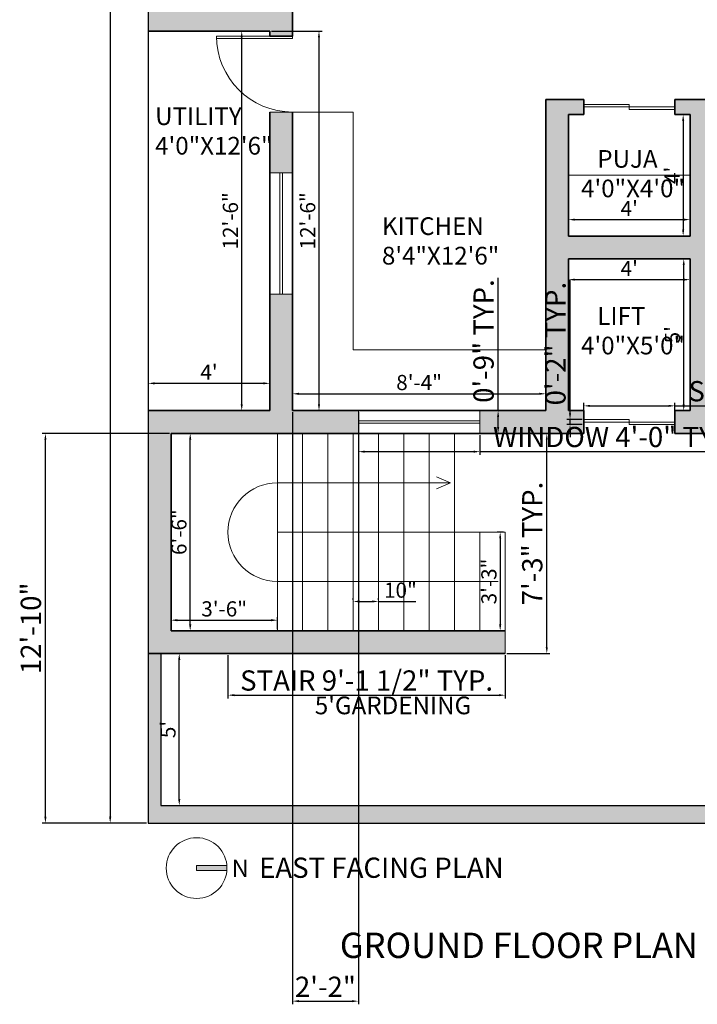
# Model space of a CAD drawing. Units: inches. Extents: x 2700 to 4052, y 1030 to 1872.
# Tile 5 of 8: x 3518 to 3786, y 1030 to 1419. Entities that reach past the tile are written whole.
import ezdxf

# ---------------------------------------------------------------- set-up
doc = ezdxf.new("R2010")
doc.units = ezdxf.units.IN
for name, color, linetype, lineweight in [('A-ANNO-DIMS', 2, 'Continuous', 13), ('A-ANNO-SYMB', 7, 'Continuous', 18), ('A-ANNO-TITL', 7, 'Continuous', 25), ('A-AREA-IDEN', 7, 'Continuous', 18), ('A-DOOR', 4, 'Continuous', 18), ('A-FLOR-CASE', 8, 'Continuous', 18), ('A-FLOR-STRS', 7, 'Continuous', 18), ('A-GLAZ', 4, 'Continuous', 18), ('A-WALL', 7, 'Continuous', 35), ('A-WALL-PATT', 7, 'Continuous', 13), ('C-PROP', 7, 'Continuous', 25)]:
    doc.layers.add(name, color=color, linetype=linetype, lineweight=lineweight)
doc.layers.add('C-SITE-PATT', color=252, linetype='Continuous', lineweight=13, true_color=0x939598)
doc.styles.get("Standard").update_dxf_attribs({"font": 'arial.ttf'})
doc.dimstyles.new('ISO-25', dxfattribs={"dimtxt": 8, "dimasz": 2.5, "dimexe": 1.25, "dimexo": 0.625, "dimtad": 1, "dimdec": 1, "dimlunit": 3, "dimtxsty": 'Standard', "dimcen": 2.5, "dimclrt": 1, "dimadec": 0, "dimazin": 0, "dimtfac": 1, "dimtdec": 1, "dimtmove": 0, "dimatfit": 3, "dimfxl": 1, "dimarcsym": 0})

# ---------------------------------------------------------------- blocks, each defined once
blk = doc.blocks.new('*D22')
at = {"layer": 'A-ANNO-DIMS', "color": 0, "lineweight": -2, "transparency": 16777216}
for p, q in [((3568.26, 1821.52), (3552.61, 1821.52)), ((3553.86, 1819.02), (3553.86, 1104.02)), ((3568.26, 1101.52), (3552.61, 1101.52))]:
    blk.add_line(p, q, dxfattribs=at)
at = {"layer": 'A-ANNO-DIMS', "color": 0, "transparency": 16777216}
for points in [[(3553.44, 1819.02), (3554.28, 1819.02), (3553.86, 1821.52)], [(3553.44, 1104.02), (3554.28, 1104.02), (3553.86, 1101.52)]]:
    blk.add_solid(points, dxfattribs=at)
at = {"layer": 'Defpoints', "color": 0, "transparency": 16777216}
for p in [(3568.88, 1821.52), (3553.86, 1101.52), (3568.88, 1101.52)]:
    blk.add_point(p, dxfattribs=at)
at = {"layer": 'A-ANNO-DIMS', "color": 0, "transparency": 16777216, "insert": (3549.15, 1461.52), "char_height": 8, "attachment_point": 5, "rotation": 90}
blk.add_mtext("60'", dxfattribs=at)
blk = doc.blocks.new('*D23')
at = {"layer": 'A-ANNO-DIMS', "color": 0, "lineweight": -2, "transparency": 16777216}
for p, q in [((3578.51, 1255.52), (3586.72, 1255.52)), ((3585.47, 1180.02), (3585.47, 1253.02)), ((3578.51, 1177.52), (3586.72, 1177.52))]:
    blk.add_line(p, q, dxfattribs=at)
at = {"layer": 'A-ANNO-DIMS', "color": 0, "transparency": 16777216}
for points in [[(3585.05, 1253.02), (3585.89, 1253.02), (3585.47, 1255.52)], [(3585.05, 1180.02), (3585.89, 1180.02), (3585.47, 1177.52)]]:
    blk.add_solid(points, dxfattribs=at)
at = {"layer": 'Defpoints', "color": 0, "transparency": 16777216}
for p in [(3577.88, 1255.52), (3585.47, 1255.52), (3577.88, 1177.52)]:
    blk.add_point(p, dxfattribs=at)
at = {"layer": 'A-ANNO-DIMS', "color": 0, "transparency": 16777216, "insert": (3581.78, 1216.52), "char_height": 6, "attachment_point": 5, "rotation": 90}
blk.add_mtext('6\'-6"', dxfattribs=at)
blk = doc.blocks.new('*D24')
at = {"layer": 'A-ANNO-DIMS', "color": 0, "lineweight": -2, "transparency": 16777216}
for p, q in [((3577.88, 1178.14), (3577.88, 1182.97)), ((3619.88, 1178.14), (3619.88, 1182.97)), ((3580.38, 1181.72), (3617.38, 1181.72))]:
    blk.add_line(p, q, dxfattribs=at)
at = {"layer": 'A-ANNO-DIMS', "color": 0, "transparency": 16777216}
for points in [[(3580.38, 1182.14), (3580.38, 1181.3), (3577.88, 1181.72)], [(3617.38, 1182.14), (3617.38, 1181.3), (3619.88, 1181.72)]]:
    blk.add_solid(points, dxfattribs=at)
at = {"layer": 'Defpoints', "color": 0, "transparency": 16777216}
for p in [(3619.88, 1181.72), (3577.88, 1177.52), (3619.88, 1177.52)]:
    blk.add_point(p, dxfattribs=at)
at = {"layer": 'A-ANNO-DIMS', "color": 0, "transparency": 16777216, "insert": (3598.88, 1185.41), "char_height": 6, "attachment_point": 5}
blk.add_mtext('3\'-6"', dxfattribs=at)
blk = doc.blocks.new('*D25')
at = {"layer": 'A-ANNO-DIMS', "color": 0, "lineweight": -2, "transparency": 16777216}
for p, q in [((3649.88, 1189.74), (3649.88, 1190.37)), ((3652.38, 1189.12), (3657.38, 1189.12)), ((3659.88, 1189.74), (3659.88, 1190.37)), ((3659.88, 1189.12), (3674.63, 1189.12))]:
    blk.add_line(p, q, dxfattribs=at)
at = {"layer": 'A-ANNO-DIMS', "color": 0, "transparency": 16777216}
for points in [[(3652.38, 1189.54), (3652.38, 1188.7), (3649.88, 1189.12)], [(3657.38, 1189.54), (3657.38, 1188.7), (3659.88, 1189.12)]]:
    blk.add_solid(points, dxfattribs=at)
at = {"layer": 'Defpoints', "color": 0, "transparency": 16777216}
for p in [(3649.88, 1189.12), (3659.88, 1189.12), (3659.88, 1189.12)]:
    blk.add_point(p, dxfattribs=at)
at = {"layer": 'A-ANNO-DIMS', "color": 0, "transparency": 16777216, "insert": (3668.5, 1192.81), "char_height": 6, "attachment_point": 5}
blk.add_mtext('10"', dxfattribs=at)
blk = doc.blocks.new('*D26')
at = {"layer": 'A-ANNO-DIMS', "color": 0, "lineweight": -2, "transparency": 16777216}
for p, q in [((3709.26, 1216.52), (3706.66, 1216.52)), ((3707.91, 1214.02), (3707.91, 1180.02)), ((3709.26, 1177.52), (3706.66, 1177.52))]:
    blk.add_line(p, q, dxfattribs=at)
at = {"layer": 'A-ANNO-DIMS', "color": 0, "transparency": 16777216}
for points in [[(3707.49, 1214.02), (3708.32, 1214.02), (3707.91, 1216.52)], [(3707.49, 1180.02), (3708.32, 1180.02), (3707.91, 1177.52)]]:
    blk.add_solid(points, dxfattribs=at)
at = {"layer": 'Defpoints', "color": 0, "transparency": 16777216}
for p in [(3709.88, 1216.52), (3707.91, 1177.52), (3709.88, 1177.52)]:
    blk.add_point(p, dxfattribs=at)
at = {"layer": 'A-ANNO-DIMS', "color": 0, "transparency": 16777216, "insert": (3704.22, 1197.02), "char_height": 6, "attachment_point": 5, "rotation": 90}
blk.add_mtext('3\'-3"', dxfattribs=at)
blk = doc.blocks.new('*D27')
at = {"layer": 'A-ANNO-DIMS', "color": 0, "lineweight": -2, "transparency": 16777216}
for p, q in [((3574.51, 1168.52), (3582.39, 1168.52)), ((3581.14, 1111.02), (3581.14, 1166.02)), ((3574.51, 1108.52), (3582.39, 1108.52))]:
    blk.add_line(p, q, dxfattribs=at)
at = {"layer": 'A-ANNO-DIMS', "color": 0, "transparency": 16777216}
for points in [[(3580.72, 1166.02), (3581.56, 1166.02), (3581.14, 1168.52)], [(3580.72, 1111.02), (3581.56, 1111.02), (3581.14, 1108.52)]]:
    blk.add_solid(points, dxfattribs=at)
at = {"layer": 'Defpoints', "color": 0, "transparency": 16777216}
for p in [(3573.88, 1168.52), (3581.14, 1168.52), (3573.88, 1108.52)]:
    blk.add_point(p, dxfattribs=at)
at = {"layer": 'A-ANNO-DIMS', "color": 0, "transparency": 16777216, "insert": (3577.46, 1138.52), "char_height": 6, "attachment_point": 5, "rotation": 90}
blk.add_mtext("5'", dxfattribs=at)
blk = doc.blocks.new('*D28')
at = {"layer": 'A-ANNO-DIMS', "color": 0, "lineweight": -2, "transparency": 16777216}
for p, q in [((3734.88, 1323.89), (3734.88, 1315.04)), ((3782.88, 1323.89), (3782.88, 1315.04)), ((3737.38, 1316.29), (3780.38, 1316.29))]:
    blk.add_line(p, q, dxfattribs=at)
at = {"layer": 'A-ANNO-DIMS', "color": 0, "transparency": 16777216}
for points in [[(3737.38, 1316.71), (3737.38, 1315.87), (3734.88, 1316.29)], [(3780.38, 1316.71), (3780.38, 1315.87), (3782.88, 1316.29)]]:
    blk.add_solid(points, dxfattribs=at)
at = {"layer": 'Defpoints', "color": 0, "transparency": 16777216}
for p in [(3734.88, 1324.52), (3782.88, 1324.52), (3782.88, 1316.29)]:
    blk.add_point(p, dxfattribs=at)
at = {"layer": 'A-ANNO-DIMS', "color": 0, "transparency": 16777216, "insert": (3758.88, 1319.91), "char_height": 6, "attachment_point": 5}
blk.add_mtext("4'", dxfattribs=at)
blk = doc.blocks.new('*D29')
at = {"layer": 'A-ANNO-DIMS', "color": 0, "lineweight": -2, "transparency": 16777216}
for p, q in [((3782.26, 1324.52), (3779.15, 1324.52)), ((3780.4, 1267.02), (3780.4, 1322.02)), ((3782.26, 1264.52), (3779.15, 1264.52))]:
    blk.add_line(p, q, dxfattribs=at)
at = {"layer": 'A-ANNO-DIMS', "color": 0, "transparency": 16777216}
for points in [[(3779.98, 1322.02), (3780.81, 1322.02), (3780.4, 1324.52)], [(3779.98, 1267.02), (3780.81, 1267.02), (3780.4, 1264.52)]]:
    blk.add_solid(points, dxfattribs=at)
at = {"layer": 'Defpoints', "color": 0, "transparency": 16777216}
for p in [(3780.4, 1324.52), (3782.88, 1324.52), (3782.88, 1264.52)]:
    blk.add_point(p, dxfattribs=at)
at = {"layer": 'A-ANNO-DIMS', "color": 0, "transparency": 16777216, "insert": (3776.72, 1294.52), "char_height": 6, "attachment_point": 5, "rotation": 90}
blk.add_mtext("5'", dxfattribs=at)
blk = doc.blocks.new('*D30')
at = {"layer": 'A-ANNO-DIMS', "color": 0, "lineweight": -2, "transparency": 16777216}
for p, q in [((3734.88, 1334.14), (3734.88, 1341.26)), ((3737.38, 1340.01), (3780.38, 1340.01)), ((3782.88, 1334.14), (3782.88, 1341.26))]:
    blk.add_line(p, q, dxfattribs=at)
at = {"layer": 'A-ANNO-DIMS', "color": 0, "transparency": 16777216}
for points in [[(3737.38, 1340.43), (3737.38, 1339.59), (3734.88, 1340.01)], [(3780.38, 1340.43), (3780.38, 1339.59), (3782.88, 1340.01)]]:
    blk.add_solid(points, dxfattribs=at)
at = {"layer": 'Defpoints', "color": 0, "transparency": 16777216}
for p in [(3782.88, 1340.01), (3734.88, 1333.52), (3782.88, 1333.52)]:
    blk.add_point(p, dxfattribs=at)
at = {"layer": 'A-ANNO-DIMS', "color": 0, "transparency": 16777216, "insert": (3758.88, 1343.63), "char_height": 6, "attachment_point": 5}
blk.add_mtext("4'", dxfattribs=at)
blk = doc.blocks.new('*D31')
at = {"layer": 'A-ANNO-DIMS', "color": 0, "lineweight": -2, "transparency": 16777216}
for p, q in [((3782.26, 1381.52), (3778.92, 1381.52)), ((3780.17, 1379.02), (3780.17, 1336.02)), ((3782.26, 1333.52), (3778.92, 1333.52))]:
    blk.add_line(p, q, dxfattribs=at)
at = {"layer": 'A-ANNO-DIMS', "color": 0, "transparency": 16777216}
for points in [[(3779.75, 1379.02), (3780.59, 1379.02), (3780.17, 1381.52)], [(3779.75, 1336.02), (3780.59, 1336.02), (3780.17, 1333.52)]]:
    blk.add_solid(points, dxfattribs=at)
at = {"layer": 'Defpoints', "color": 0, "transparency": 16777216}
for p in [(3782.88, 1381.52), (3780.17, 1333.52), (3782.88, 1333.52)]:
    blk.add_point(p, dxfattribs=at)
at = {"layer": 'A-ANNO-DIMS', "color": 0, "transparency": 16777216, "insert": (3776.55, 1357.52), "char_height": 6, "attachment_point": 5, "rotation": 90}
blk.add_mtext("4'", dxfattribs=at)
blk = doc.blocks.new('*D32')
at = {"layer": 'A-ANNO-DIMS', "color": 0, "lineweight": -2, "transparency": 16777216}
for p, q in [((3625.88, 1265.14), (3625.88, 1272.43)), ((3725.88, 1265.14), (3725.88, 1272.43)), ((3628.38, 1271.18), (3723.38, 1271.18))]:
    blk.add_line(p, q, dxfattribs=at)
at = {"layer": 'A-ANNO-DIMS', "color": 0, "transparency": 16777216}
for points in [[(3628.38, 1271.6), (3628.38, 1270.77), (3625.88, 1271.18)], [(3723.38, 1271.6), (3723.38, 1270.77), (3725.88, 1271.18)]]:
    blk.add_solid(points, dxfattribs=at)
at = {"layer": 'Defpoints', "color": 0, "transparency": 16777216}
for p in [(3725.88, 1271.18), (3625.88, 1264.52), (3725.88, 1264.52)]:
    blk.add_point(p, dxfattribs=at)
at = {"layer": 'A-ANNO-DIMS', "color": 0, "transparency": 16777216, "insert": (3675.88, 1274.87), "char_height": 6, "attachment_point": 5}
blk.add_mtext('8\'-4"', dxfattribs=at)
blk = doc.blocks.new('*D33')
at = {"layer": 'A-ANNO-DIMS', "color": 0, "lineweight": -2, "transparency": 16777216}
for p, q in [((3568.88, 1276.23), (3568.88, 1274.06)), ((3616.88, 1276.23), (3616.88, 1274.06)), ((3614.38, 1275.31), (3571.38, 1275.31))]:
    blk.add_line(p, q, dxfattribs=at)
at = {"layer": 'A-ANNO-DIMS', "color": 0, "transparency": 16777216}
for points in [[(3571.38, 1275.73), (3571.38, 1274.9), (3568.88, 1275.31)], [(3614.38, 1275.73), (3614.38, 1274.9), (3616.88, 1275.31)]]:
    blk.add_solid(points, dxfattribs=at)
at = {"layer": 'Defpoints', "color": 0, "transparency": 16777216}
for p in [(3568.88, 1276.85), (3616.88, 1276.85), (3568.88, 1275.31)]:
    blk.add_point(p, dxfattribs=at)
at = {"layer": 'A-ANNO-DIMS', "color": 0, "transparency": 16777216, "insert": (3592.88, 1278.94), "char_height": 6, "attachment_point": 5}
blk.add_mtext("4'", dxfattribs=at)
blk = doc.blocks.new('*D34')
at = {"layer": 'A-ANNO-DIMS', "color": 0, "lineweight": -2, "transparency": 16777216}
for p, q in [((3593.51, 1414.52), (3607.06, 1414.52)), ((3605.81, 1267.02), (3605.81, 1412.02)), ((3596.11, 1264.52), (3607.06, 1264.52))]:
    blk.add_line(p, q, dxfattribs=at)
at = {"layer": 'A-ANNO-DIMS', "color": 0, "transparency": 16777216}
for points in [[(3605.39, 1412.02), (3606.22, 1412.02), (3605.81, 1414.52)], [(3605.39, 1267.02), (3606.22, 1267.02), (3605.81, 1264.52)]]:
    blk.add_solid(points, dxfattribs=at)
at = {"layer": 'Defpoints', "color": 0, "transparency": 16777216}
for p in [(3592.88, 1414.52), (3605.81, 1414.52), (3595.49, 1264.52)]:
    blk.add_point(p, dxfattribs=at)
at = {"layer": 'A-ANNO-DIMS', "color": 0, "transparency": 16777216, "insert": (3602.12, 1339.52), "char_height": 6, "attachment_point": 5, "rotation": 90}
blk.add_mtext('12\'-6"', dxfattribs=at)
blk = doc.blocks.new('*D35')
at = {"layer": 'A-ANNO-DIMS', "color": 0, "lineweight": -2, "transparency": 16777216}
for p, q in [((3617.51, 1414.52), (3637.58, 1414.52)), ((3636.33, 1412.02), (3636.33, 1267.02)), ((3626.51, 1264.52), (3637.58, 1264.52))]:
    blk.add_line(p, q, dxfattribs=at)
at = {"layer": 'A-ANNO-DIMS', "color": 0, "transparency": 16777216}
for points in [[(3635.91, 1412.02), (3636.74, 1412.02), (3636.33, 1414.52)], [(3635.91, 1267.02), (3636.74, 1267.02), (3636.33, 1264.52)]]:
    blk.add_solid(points, dxfattribs=at)
at = {"layer": 'Defpoints', "color": 0, "transparency": 16777216}
for p in [(3616.88, 1414.52), (3625.88, 1264.52), (3636.33, 1264.52)]:
    blk.add_point(p, dxfattribs=at)
at = {"layer": 'A-ANNO-DIMS', "color": 0, "transparency": 16777216, "insert": (3632.64, 1339.52), "char_height": 6, "attachment_point": 5, "rotation": 90}
blk.add_mtext('12\'-6"', dxfattribs=at)
blk = doc.blocks.new('DOOR-SWING-30IN')
for p, q in [((-1, 30), (-1, 0)), ((0, 30), (0, 0)), ((0, 0), (-1, 0))]:
    blk.add_line(p, q)
blk.add_arc((0, 0), 30, 90, 180)
blk = doc.blocks.new('DOOR-SLIDING-36IN')
for p, q in [((18, 2), (0, 2)), ((36, 1), (0, 1)), ((18, 2), (18, 0)), ((36, 0), (18, 0))]:
    blk.add_line(p, q)
blk = doc.blocks.new('WINDOW-48IN')
for p, q in [((-24, -4.5), (-24, 4.5)), ((24, -4.5), (24, 4.5)), ((-24, 0.5), (24, 0.5)), ((-24, -0.5), (24, -0.5))]:
    blk.add_line(p, q)
blk = doc.blocks.new('STAIR-RETURN-FLIGHT')
for p, q in [((19.5, 87), (19.5, 9)), ((29.5, 87), (29.5, 9)), ((39.5, 87), (39.5, 9)), ((49.5, 87), (49.5, 9)), ((59.5, 87), (59.5, 9)), ((69.5, 87), (69.5, 9)), ((79.5, 87), (79.5, 9)), ((89.5, 87), (89.5, 9)), ((87.91, 67.5), (82.37, 69.91)), ((87.91, 67.5), (82.37, 65.09)), ((109.5, 48), (19.5, 48)), ((99.5, 48), (99.5, 9)), ((109.5, 48), (109.5, 0))]:
    blk.add_line(p, q)
blk.add_lwpolyline([(106.75, 28.5), (19.5, 28.5, -1), (19.5, 67.5), (87.91, 67.5)], format="xyb")
blk = doc.blocks.new('NORTH-INDICATOR')
at = {"transparency": 33554687}
h = blk.add_hatch(color=256, dxfattribs=at)
h.dxf.hatch_style = 1
h.paths.add_polyline_path([(0, 1), (0, -1), (11.96, -1, 0.020861), (12, 0, 0.020861), (11.96, 1)])
for p, q in [((0, -1), (0, 1)), ((0, 1), (11.96, 1)), ((12, -1), (0, -1))]:
    blk.add_line(p, q)
blk.add_circle((0, 0), 12)
blk.add_text('N', height=6.9).set_placement((13.83, -3.53))
blk = doc.blocks.new('*D64')
at = {"layer": 'A-ANNO-DIMS', "color": 0, "lineweight": -2, "transparency": 16777216}
for p, q in [((3651.88, 1254.89), (3651.88, 1247.07)), ((3699.88, 1254.89), (3699.88, 1247.07)), ((3654.38, 1248.32), (3697.38, 1248.32)), ((3699.88, 1248.32), (3804.87, 1248.32))]:
    blk.add_line(p, q, dxfattribs=at)
at = {"layer": 'A-ANNO-DIMS', "color": 0, "transparency": 16777216}
for points in [[(3654.38, 1248.73), (3654.38, 1247.9), (3651.88, 1248.32)], [(3697.38, 1248.73), (3697.38, 1247.9), (3699.88, 1248.32)]]:
    blk.add_solid(points, dxfattribs=at)
at = {"layer": 'Defpoints', "color": 0, "transparency": 16777216}
for p in [(3651.88, 1255.52), (3699.88, 1255.52), (3699.88, 1248.32)]:
    blk.add_point(p, dxfattribs=at)
at = {"layer": 'A-ANNO-DIMS', "color": 1, "transparency": 16777216, "insert": (3753.62, 1253.08), "char_height": 8, "attachment_point": 5}
blk.add_mtext('WINDOW 4\'-0" TYP.', dxfattribs=at)
blk = doc.blocks.new('*D65')
at = {"layer": 'A-ANNO-DIMS', "color": 0, "lineweight": -2, "transparency": 16777216}
for p, q in [((3707.08, 1264.52), (3707.08, 1317.03)), ((3700.51, 1264.52), (3708.33, 1264.52)), ((3707.08, 1258.02), (3707.08, 1262.02)), ((3700.51, 1255.52), (3708.33, 1255.52))]:
    blk.add_line(p, q, dxfattribs=at)
at = {"layer": 'A-ANNO-DIMS', "color": 0, "transparency": 16777216}
for points in [[(3706.67, 1262.02), (3707.5, 1262.02), (3707.08, 1264.52)], [(3706.67, 1258.02), (3707.5, 1258.02), (3707.08, 1255.52)]]:
    blk.add_solid(points, dxfattribs=at)
at = {"layer": 'Defpoints', "color": 0, "transparency": 16777216}
for p in [(3699.88, 1264.52), (3707.08, 1264.52), (3699.88, 1255.52)]:
    blk.add_point(p, dxfattribs=at)
at = {"layer": 'A-ANNO-DIMS', "color": 1, "transparency": 16777216, "insert": (3702.37, 1292.02), "char_height": 8, "attachment_point": 5, "rotation": 90}
blk.add_mtext('0\'-9" TYP.', dxfattribs=at)
blk = doc.blocks.new('*D76')
at = {"layer": 'A-ANNO-DIMS', "color": 0, "lineweight": -2, "transparency": 16777216}
for p, q in [((3740.88, 1261.64), (3740.88, 1267.67)), ((3743.38, 1266.42), (3774.38, 1266.42)), ((3776.88, 1261.64), (3776.88, 1267.67)), ((3776.88, 1266.42), (3872.83, 1266.42))]:
    blk.add_line(p, q, dxfattribs=at)
at = {"layer": 'A-ANNO-DIMS', "color": 0, "transparency": 16777216}
for points in [[(3743.38, 1266.83), (3743.38, 1266), (3740.88, 1266.42)], [(3774.38, 1266.83), (3774.38, 1266), (3776.88, 1266.42)]]:
    blk.add_solid(points, dxfattribs=at)
at = {"layer": 'Defpoints', "color": 0, "transparency": 16777216}
for p in [(3776.88, 1266.42), (3740.88, 1261.02), (3776.88, 1261.02)]:
    blk.add_point(p, dxfattribs=at)
at = {"layer": 'A-ANNO-DIMS', "color": 1, "transparency": 16777216, "insert": (3826.11, 1271.18), "char_height": 8, "attachment_point": 5}
blk.add_mtext('SLIDER 3\'-0" TYP.', dxfattribs=at)
blk = doc.blocks.new('*D77')
at = {"layer": 'A-ANNO-DIMS', "color": 0, "lineweight": -2, "transparency": 16777216}
for p, q in [((3735.48, 1263.52), (3735.48, 1316.03)), ((3740.26, 1261.02), (3734.23, 1261.02)), ((3735.48, 1259.02), (3735.48, 1261.02)), ((3740.26, 1259.02), (3734.23, 1259.02)), ((3735.48, 1256.52), (3735.48, 1254.02))]:
    blk.add_line(p, q, dxfattribs=at)
at = {"layer": 'A-ANNO-DIMS', "color": 0, "transparency": 16777216}
for points in [[(3735.07, 1263.52), (3735.9, 1263.52), (3735.48, 1261.02)], [(3735.07, 1256.52), (3735.9, 1256.52), (3735.48, 1259.02)]]:
    blk.add_solid(points, dxfattribs=at)
at = {"layer": 'Defpoints', "color": 0, "transparency": 16777216}
for p in [(3735.48, 1261.02), (3740.88, 1261.02), (3740.88, 1259.02)]:
    blk.add_point(p, dxfattribs=at)
at = {"layer": 'A-ANNO-DIMS', "color": 1, "transparency": 16777216, "insert": (3730.77, 1291.02), "char_height": 8, "attachment_point": 5, "rotation": 90}
blk.add_mtext('0\'-2" TYP.', dxfattribs=at)
blk = doc.blocks.new('*D80')
at = {"layer": 'A-ANNO-DIMS', "color": 0, "lineweight": -2, "transparency": 16777216}
for p, q in [((3600.38, 1167.89), (3600.38, 1150.84)), ((3709.88, 1167.89), (3709.88, 1150.84)), ((3602.88, 1152.09), (3707.38, 1152.09))]:
    blk.add_line(p, q, dxfattribs=at)
at = {"layer": 'A-ANNO-DIMS', "color": 0, "transparency": 16777216}
for points in [[(3602.88, 1152.51), (3602.88, 1151.68), (3600.38, 1152.09)], [(3707.38, 1152.51), (3707.38, 1151.68), (3709.88, 1152.09)]]:
    blk.add_solid(points, dxfattribs=at)
at = {"layer": 'Defpoints', "color": 0, "transparency": 16777216}
for p in [(3600.38, 1168.52), (3709.88, 1168.52), (3709.88, 1152.09)]:
    blk.add_point(p, dxfattribs=at)
at = {"layer": 'A-ANNO-DIMS', "color": 1, "transparency": 16777216, "insert": (3655.13, 1156.85), "char_height": 8, "attachment_point": 5}
blk.add_mtext('STAIR 9\'-1 1/2" TYP.', dxfattribs=at)
blk = doc.blocks.new('*D81')
at = {"layer": 'A-ANNO-DIMS', "color": 0, "lineweight": -2, "transparency": 16777216}
for p, q in [((3710.51, 1255.52), (3727.56, 1255.52)), ((3726.31, 1171.02), (3726.31, 1253.02)), ((3710.51, 1168.52), (3727.56, 1168.52))]:
    blk.add_line(p, q, dxfattribs=at)
at = {"layer": 'A-ANNO-DIMS', "color": 0, "transparency": 16777216}
for points in [[(3725.89, 1253.02), (3726.72, 1253.02), (3726.31, 1255.52)], [(3725.89, 1171.02), (3726.72, 1171.02), (3726.31, 1168.52)]]:
    blk.add_solid(points, dxfattribs=at)
at = {"layer": 'Defpoints', "color": 0, "transparency": 16777216}
for p in [(3709.88, 1255.52), (3726.31, 1255.52), (3709.88, 1168.52)]:
    blk.add_point(p, dxfattribs=at)
at = {"layer": 'A-ANNO-DIMS', "color": 1, "transparency": 16777216, "insert": (3721.6, 1212.02), "char_height": 8, "attachment_point": 5, "rotation": 90}
blk.add_mtext('7\'-3" TYP.', dxfattribs=at)
blk = doc.blocks.new('*D105')
at = {"layer": 'A-ANNO-DIMS', "color": 0, "lineweight": -2, "transparency": 16777216}
for p, q in [((3577.26, 1255.52), (3527.03, 1255.52)), ((3528.28, 1104.02), (3528.28, 1253.02)), ((3568.26, 1101.52), (3527.03, 1101.52))]:
    blk.add_line(p, q, dxfattribs=at)
at = {"layer": 'A-ANNO-DIMS', "color": 0, "transparency": 16777216}
for points in [[(3527.87, 1253.02), (3528.7, 1253.02), (3528.28, 1255.52)], [(3527.87, 1104.02), (3528.7, 1104.02), (3528.28, 1101.52)]]:
    blk.add_solid(points, dxfattribs=at)
at = {"layer": 'Defpoints', "color": 0, "transparency": 16777216}
for p in [(3528.28, 1255.52), (3577.88, 1255.52), (3568.88, 1101.52)]:
    blk.add_point(p, dxfattribs=at)
at = {"layer": 'A-ANNO-DIMS', "color": 1, "transparency": 16777216, "insert": (3523.57, 1178.52), "char_height": 8, "attachment_point": 5, "rotation": 90}
blk.add_mtext('12\'-10"', dxfattribs=at)
blk = doc.blocks.new('*D113')
at = {"layer": 'A-ANNO-DIMS', "color": 0, "lineweight": -2, "transparency": 16777216}
for p, q in [((3625.88, 1263.89), (3625.88, 1029.93)), ((3651.88, 1263.89), (3651.88, 1029.93)), ((3628.38, 1031.18), (3649.38, 1031.18))]:
    blk.add_line(p, q, dxfattribs=at)
at = {"layer": 'A-ANNO-DIMS', "color": 0, "transparency": 16777216}
for points in [[(3628.38, 1031.6), (3628.38, 1030.77), (3625.88, 1031.18)], [(3649.38, 1031.6), (3649.38, 1030.77), (3651.88, 1031.18)]]:
    blk.add_solid(points, dxfattribs=at)
at = {"layer": 'Defpoints', "color": 0, "transparency": 16777216}
for p in [(3625.88, 1264.52), (3651.88, 1264.52), (3651.88, 1031.18)]:
    blk.add_point(p, dxfattribs=at)
at = {"layer": 'A-ANNO-DIMS', "color": 1, "transparency": 16777216, "insert": (3638.88, 1035.82), "char_height": 8, "attachment_point": 5}
blk.add_mtext('2\'-2"', dxfattribs=at)

msp = doc.modelspace()

# ---------------------------------------------------------------- hatches: boundary and pattern name
at = {"layer": 'A-WALL-PATT'}
h = msp.add_hatch(color=256, dxfattribs=at)
h.dxf.hatch_style = 1
h.paths.add_polyline_path([(3904.88, 1539.52), (3895.88, 1539.52), (3895.88, 1479.52), (3904.88, 1479.52)])
h.paths.add_polyline_path([(3904.88, 1666.52), (3895.88, 1666.52), (3895.88, 1636.52), (3760.88, 1636.52), (3760.88, 1638.52), (3751.88, 1638.52), (3751.88, 1627.52), (3868.81, 1627.52, -0.035851), (3872.34, 1627.52), (3895.88, 1627.52), (3895.88, 1599.52), (3904.88, 1599.52)])
h.paths.add_polyline_path([(3595.88, 1537.52), (3586.88, 1537.52), (3586.88, 1486.52), (3595.88, 1486.52), (3595.88, 1501.52), (3677.88, 1501.52), (3677.88, 1507.52), (3595.88, 1507.52)], flags=17)
h.paths.add_polyline_path([(3595.88, 1438.52), (3586.88, 1438.52), (3586.88, 1423.52), (3568.88, 1423.52), (3568.88, 1414.52), (3616.88, 1414.52), (3616.88, 1412.52), (3625.88, 1412.52), (3625.88, 1423.52), (3595.88, 1423.52)])
h.paths.add_polyline_path([(3721.88, 1636.52), (3706.88, 1636.52), (3706.88, 1638.52), (3697.88, 1638.52), (3697.88, 1636.52), (3595.88, 1636.52), (3595.88, 1685.52), (3586.88, 1685.52), (3586.88, 1597.52), (3595.88, 1597.52), (3595.88, 1627.52), (3715.88, 1627.52), (3715.88, 1507.52), (3713.88, 1507.52), (3713.88, 1501.52), (3715.88, 1501.52), (3715.88, 1453.52), (3721.88, 1453.52)])
h.paths.add_polyline_path([(3724.88, 1756.52), (3863.88, 1756.52), (3863.88, 1762.52), (3814.88, 1762.52), (3814.88, 1812.52), (3895.88, 1812.52), (3895.88, 1799.52), (3904.88, 1799.52), (3904.88, 1821.52), (3796.88, 1821.52), (3796.88, 1812.52), (3808.88, 1812.52), (3808.88, 1762.52), (3724.88, 1762.52), (3724.88, 1764.52), (3715.88, 1764.52), (3715.88, 1686.52), (3697.88, 1686.52), (3697.88, 1674.52), (3706.88, 1674.52), (3706.88, 1677.52), (3751.88, 1677.52), (3751.88, 1674.52), (3760.88, 1674.52), (3760.88, 1686.52), (3724.88, 1686.52)])
h.paths.add_polyline_path([(3904.88, 1775.52), (3895.88, 1775.52), (3895.88, 1762.52), (3893.88, 1762.52), (3893.88, 1756.52), (3895.88, 1756.52), (3895.88, 1726.52), (3904.88, 1726.52)], flags=17)
h.paths.add_polyline_path([(3772.88, 1821.52), (3586.88, 1821.52), (3586.88, 1745.52), (3595.88, 1745.52), (3595.88, 1812.52), (3715.88, 1812.52), (3715.88, 1794.52), (3724.88, 1794.52), (3724.88, 1812.52), (3772.88, 1812.52)])
h = msp.add_hatch(color=256, dxfattribs=at)
h.dxf.hatch_style = 1
h.paths.add_polyline_path([(3651.88, 1264.52), (3625.88, 1264.52), (3625.88, 1310.49), (3616.88, 1310.49), (3616.88, 1304.37), (3616.88, 1264.52), (3568.88, 1264.52), (3568.88, 1168.52), (3709.88, 1168.52), (3709.88, 1177.52), (3577.88, 1177.52), (3577.88, 1255.52), (3651.88, 1255.52)])
h.paths.add_polyline_path([(3740.88, 1264.52), (3734.88, 1264.52), (3734.88, 1324.52), (3782.88, 1324.52), (3782.88, 1264.52), (3776.88, 1264.52), (3776.88, 1255.52), (3791.88, 1255.52), (3791.88, 1378.52), (3794.88, 1378.52), (3794.88, 1387.52), (3776.88, 1387.52), (3776.88, 1381.52), (3782.88, 1381.52), (3782.88, 1333.52), (3734.88, 1333.52), (3734.88, 1381.52), (3740.88, 1381.52), (3740.88, 1387.52), (3725.88, 1387.52), (3725.88, 1264.52), (3699.88, 1264.52), (3699.88, 1255.52), (3740.88, 1255.52)])
h.paths.add_polyline_path([(3625.88, 1382.52), (3616.88, 1382.52), (3616.88, 1358.49), (3625.88, 1358.49)])
h.paths.add_polyline_path([(3845.88, 1387.52), (3842.88, 1387.52), (3842.88, 1378.52), (3845.88, 1378.52)])
h.paths.add_polyline_path([(3904.88, 1431.52), (3895.88, 1431.52), (3895.88, 1387.52), (3893.88, 1387.52), (3893.88, 1378.52), (3895.88, 1378.52), (3895.88, 1300.52), (3904.88, 1300.52)])
h.paths.add_polyline_path([(3584.49, 1565.14), (3584.49, 1604.05), (3576.25, 1604.05), (3576.25, 1565.14)], flags=9)
h.paths.add_polyline_path([(3711.56, 1565.68), (3711.56, 1611.46), (3703.32, 1611.46), (3703.32, 1565.68)], flags=9)
h.paths.add_polyline_path([(3737.75, 1697.89), (3737.75, 1743.66), (3729.51, 1743.66), (3729.51, 1697.89)], flags=9)
h.paths.add_polyline_path([(3633.29, 1800.61), (3679.06, 1800.61), (3679.06, 1808.85), (3633.29, 1808.85)], flags=9)
h.paths.add_polyline_path([(3569.7, 1361.72), (3618.67, 1361.72), (3618.67, 1388.34), (3569.7, 1388.34)], flags=9)
h.paths.add_polyline_path([(3658.81, 1318.27), (3708.12, 1318.27), (3708.12, 1344.89), (3658.81, 1344.89)], flags=9)
h.paths.add_polyline_path([(3791.11, 1507.34), (3845.25, 1507.34), (3845.25, 1533.96), (3791.11, 1533.96)], flags=9)
h.paths.add_polyline_path([(3744.61, 1774.23), (3794.63, 1774.23), (3794.63, 1800.84), (3744.61, 1800.84)], flags=9)
h.paths.add_polyline_path([(3831.1, 1774.23), (3881.17, 1774.23), (3881.17, 1800.84), (3831.1, 1800.84)], flags=9)
h.paths.add_polyline_path([(3791.11, 1664.37), (3855.09, 1664.37), (3855.09, 1690.98), (3791.11, 1690.98)], flags=9)
h.paths.add_polyline_path([(3626.06, 1747.79), (3690.04, 1747.79), (3690.04, 1774.41), (3626.06, 1774.41)], flags=9)
h.paths.add_polyline_path([(3626.06, 1590.97), (3690.04, 1590.97), (3690.04, 1617.58), (3626.06, 1617.58)], flags=9)
h.paths.add_polyline_path([(3616.71, 1447.4), (3665.68, 1447.4), (3665.68, 1474.01), (3616.71, 1474.01)], flags=9)
at = {"layer": 'C-SITE-PATT'}
h = msp.add_hatch(color=256, dxfattribs=at)
h.dxf.hatch_style = 1
h.paths.add_polyline_path([(3573.88, 1821.52), (3568.88, 1821.52), (3568.88, 1423.52), (3573.88, 1423.52)])
h.paths.add_polyline_path([(3791.88, 1108.52), (3573.88, 1108.52), (3573.88, 1168.52), (3568.88, 1168.52), (3568.88, 1101.52), (3791.88, 1101.52)])
h.paths.add_polyline_path([(3928.88, 1821.52), (3923.88, 1821.52), (3923.88, 1108.52), (3911.88, 1108.52), (3911.88, 1101.52), (3928.88, 1101.52)])

# ---------------------------------------------------------------- linework, layer by layer
at = {"layer": 'A-FLOR-CASE'}
for p, q in [((3649.88, 1382.52), (3616.88, 1382.52)), ((3649.88, 1288.52), (3649.88, 1382.52)), ((3782.88, 1357.52), (3734.88, 1357.52)), ((3725.88, 1288.52), (3649.88, 1288.52))]:
    msp.add_line(p, q, dxfattribs=at)
at = {"layer": 'A-WALL'}
for p, q in [((3625.88, 1412.52), (3625.88, 1423.52)), ((3616.88, 1414.52), (3568.88, 1414.52)), ((3616.88, 1412.52), (3616.88, 1414.52)), ((3625.88, 1412.52), (3616.88, 1412.52)), ((3740.88, 1387.52), (3725.88, 1387.52)), ((3725.88, 1264.52), (3725.88, 1387.52)), ((3740.88, 1381.52), (3740.88, 1387.52)), ((3845.88, 1387.52), (3776.88, 1387.52)), ((3776.88, 1381.52), (3776.88, 1387.52)), ((3616.88, 1264.52), (3616.88, 1382.52)), ((3625.88, 1264.52), (3625.88, 1382.52)), ((3740.88, 1381.52), (3734.88, 1381.52)), ((3734.88, 1333.52), (3734.88, 1381.52)), ((3782.88, 1381.52), (3776.88, 1381.52)), ((3782.88, 1333.52), (3782.88, 1381.52)), ((3782.88, 1333.52), (3734.88, 1333.52)), ((3782.88, 1324.52), (3734.88, 1324.52)), ((3734.88, 1264.52), (3734.88, 1324.52)), ((3782.88, 1264.52), (3782.88, 1324.52)), ((3616.88, 1264.52), (3568.88, 1264.52)), ((3725.88, 1264.52), (3625.88, 1264.52)), ((3740.88, 1264.52), (3734.88, 1264.52)), ((3740.88, 1255.52), (3740.88, 1264.52)), ((3782.88, 1264.52), (3776.88, 1264.52)), ((3776.88, 1255.52), (3776.88, 1264.52)), ((3740.88, 1255.52), (3577.88, 1255.52)), ((3577.88, 1255.52), (3577.88, 1177.52)), ((3791.88, 1255.52), (3776.88, 1255.52)), ((3709.88, 1177.52), (3577.88, 1177.52)), ((3709.88, 1168.52), (3568.88, 1168.52))]:
    msp.add_line(p, q, dxfattribs=at)
at = {"layer": 'C-PROP'}
for p, q in [((3568.88, 1264.52), (3568.88, 1101.52)), ((3573.88, 1168.52), (3573.88, 1108.52)), ((3573.88, 1108.52), (3791.88, 1108.52))]:
    msp.add_line(p, q, dxfattribs=at)
msp.add_lwpolyline([(3911.88, 1101.52), (3928.88, 1101.52), (3928.88, 1821.52), (3568.88, 1821.52), (3568.88, 1101.52), (3791.88, 1101.52)], dxfattribs=at)

# ---------------------------------------------------------------- block references
at = {"layer": 'A-ANNO-SYMB'}
msp.add_blockref('NORTH-INDICATOR', (3587.98, 1083.78), dxfattribs=at)
at = {"layer": 'A-DOOR'}
for name, p, rotation in [('DOOR-SWING-30IN', (3625.88, 1412.52), 90.00000000000067), ('DOOR-SLIDING-36IN', (3776.88, 1385.52), 180)]:
    msp.add_blockref(name, p, dxfattribs=dict(at, rotation=rotation))
msp.add_blockref('DOOR-SLIDING-36IN', (3740.88, 1259.02), dxfattribs=at)
at = {"layer": 'A-FLOR-STRS'}
msp.add_blockref('STAIR-RETURN-FLIGHT', (3600.38, 1168.52), dxfattribs=at)
at = {"layer": 'A-GLAZ', "rotation": 90.00000000000364}
msp.add_blockref('WINDOW-48IN', (3621.38, 1334.49), dxfattribs=at)
at = {"layer": 'A-GLAZ'}
msp.add_blockref('WINDOW-48IN', (3675.88, 1260.02), dxfattribs=at)

# ---------------------------------------------------------------- texts
at = {"layer": 'A-ANNO-TITL', "attachment_point": 1}
for s, insert, char_height in [('{\\fTimes New Roman|b0|i0|c0|p18;EAST FACING PLAN}', (3612.67, 1087.91), 8), ('{\\fTimes New Roman|b0|i0|c0|p18;GROUND FLOOR PLAN}', (3644.57, 1058.23), 10)]:
    msp.add_mtext_dynamic_manual_height_columns(s, width=196.2607, gutter_width=12.5, heights=[0], dxfattribs=dict(at, insert=insert, char_height=char_height))
at = {"layer": 'A-AREA-IDEN', "char_height": 7, "attachment_point": 1}
for s, insert in [('{\\fTimes New Roman|b0|i0|c0|p18;UTILITY\\P4\'0"X12\'6"}', (3571.61, 1384.37)), ('{\\fTimes New Roman|b0|i0|c0|p18;   PUJA\\P4\'0"X4\'0"}', (3739.84, 1367.51)), ('{\\fTimes New Roman|b0|i0|c0|p18;KITCHEN\\P8\'4"X12\'6"}', (3661.19, 1340.93)), ('{\\fTimes New Roman|b0|i0|c0|p18;   LIFT\\P4\'0"X5\'0"}', (3739.84, 1305.42)), ("{\\fTimes New Roman|b0|i0|c0|p18; 5'GARDENING}", (3634.68, 1151.55))]:
    msp.add_mtext_dynamic_manual_height_columns(s, width=61.0557, gutter_width=12.5, heights=[0], dxfattribs=dict(at, insert=insert))

# ---------------------------------------------------------------- dimensions: what is measured, and where the dimension line sits
at = {"layer": 'A-ANNO-DIMS'}
for base, p1, p2, angle, override, picture, middle in [((3553.86, 1101.52), (3568.88, 1821.52), (3568.88, 1101.52), 90, {"dimclrd": 0, "dimclre": 0, "dimclrt": 0}, '*D22', (3549.15, 1461.52)), ((3605.81, 1414.52), (3595.49, 1264.52), (3592.88, 1414.52), 90, {"dimtxt": 6, "dimclrd": 0, "dimclre": 0, "dimclrt": 0}, '*D34', (3602.12, 1339.52)), ((3636.33, 1264.52), (3616.88, 1414.52), (3625.88, 1264.52), 90, {"dimtxt": 6, "dimclrd": 0, "dimclre": 0, "dimclrt": 0}, '*D35', (3632.64, 1339.52)), ((3780.17, 1333.52), (3782.88, 1381.52), (3782.88, 1333.52), 90, {"dimtxt": 6, "dimclrd": 0, "dimclre": 0, "dimclrt": 0}, '*D31', (3776.55, 1357.52)), ((3780.4, 1324.52), (3782.88, 1264.52), (3782.88, 1324.52), 270, {"dimtxt": 6, "dimclrd": 0, "dimclre": 0, "dimclrt": 0}, '*D29', (3776.72, 1294.52)), ((3528.28, 1255.52), (3568.88, 1101.52), (3577.88, 1255.52), 90, {"dimdec": 1, "dimlfac": 1, "dimrnd": 0, "dimzin": 1, "dimdsep": 46, "dimlunit": 4, "dimfrac": 2}, '*D105', (3523.57, 1178.52)), ((3585.47, 1255.52), (3577.88, 1177.52), (3577.88, 1255.52), 270, {"dimtxt": 6, "dimclrd": 0, "dimclre": 0, "dimclrt": 0}, '*D23', (3581.78, 1216.52)), ((3707.91, 1177.52), (3709.88, 1216.52), (3709.88, 1177.52), 90, {"dimtxt": 6, "dimclrd": 0, "dimclre": 0, "dimclrt": 0}, '*D26', (3704.22, 1197.02)), ((3581.14, 1168.52), (3573.88, 1108.52), (3573.88, 1168.52), 270, {"dimtxt": 6, "dimclrd": 0, "dimclre": 0, "dimclrt": 0}, '*D27', (3577.46, 1138.52))]:
    dim = msp.add_linear_dim(base=base, p1=p1, p2=p2, angle=angle, dimstyle='ISO-25', override=override, dxfattribs=at)
    dim.commit()
    dim.dimension.update_dxf_attribs({"geometry": picture, "text_midpoint": middle})
for base, p1, p2, override, picture, middle in [((3782.88, 1340.01), (3734.88, 1333.52), (3782.88, 1333.52), {"dimtxt": 6, "dimclrd": 0, "dimclre": 0, "dimclrt": 0}, '*D30', (3758.88, 1343.63)), ((3782.88, 1316.29), (3734.88, 1324.52), (3782.88, 1324.52), {"dimtxt": 6, "dimclrd": 0, "dimclre": 0, "dimclrt": 0}, '*D28', (3758.88, 1319.91)), ((3568.88, 1275.31), (3616.88, 1276.85), (3568.88, 1276.85), {"dimtxt": 6, "dimclrd": 0, "dimclre": 0, "dimclrt": 0}, '*D33', (3592.88, 1278.94)), ((3725.88, 1271.18), (3625.88, 1264.52), (3725.88, 1264.52), {"dimtxt": 6, "dimclrd": 0, "dimclre": 0, "dimclrt": 0}, '*D32', (3675.88, 1274.87)), ((3651.88, 1031.18), (3625.88, 1264.52), (3651.88, 1264.52), {"dimdec": 1, "dimlfac": 1, "dimrnd": 0, "dimzin": 1, "dimdsep": 46, "dimlunit": 4, "dimfrac": 2}, '*D113', (3638.88, 1035.82)), ((3659.88, 1189.12), (3649.88, 1189.12), (3659.88, 1189.12), {"dimtxt": 6, "dimclrd": 0, "dimclre": 0, "dimclrt": 0}, '*D25', (3668.5, 1192.81)), ((3619.88, 1181.72), (3577.88, 1177.52), (3619.88, 1177.52), {"dimtxt": 6, "dimclrd": 0, "dimclre": 0, "dimclrt": 0}, '*D24', (3598.88, 1185.41))]:
    dim = msp.add_linear_dim(base=base, p1=p1, p2=p2, dimstyle='ISO-25', override=override, dxfattribs=at)
    dim.commit()
    dim.dimension.update_dxf_attribs({"geometry": picture, "text_midpoint": middle})
for base, p1, p2, picture, middle in [((3707.08, 1264.52), (3699.88, 1255.52), (3699.88, 1264.52), '*D65', (3702.37, 1292.02)), ((3735.48, 1261.02), (3740.88, 1259.02), (3740.88, 1261.02), '*D77', (3730.77, 1291.02)), ((3726.31, 1255.52), (3709.88, 1168.52), (3709.88, 1255.52), '*D81', (3721.6, 1212.02))]:
    dim = msp.add_linear_dim(base=base, p1=p1, p2=p2, angle=90, text='<> TYP.', dimstyle='ISO-25', override={"dimdec": 1, "dimlfac": 1, "dimrnd": 0, "dimzin": 1, "dimdsep": 46, "dimlunit": 4, "dimfrac": 2}, dxfattribs=at)
    dim.commit()
    dim.dimension.update_dxf_attribs({"geometry": picture, "text_midpoint": middle})
for base, p1, p2, text, picture, middle in [((3776.88, 1266.42), (3740.88, 1261.02), (3776.88, 1261.02), 'SLIDER <> TYP.', '*D76', (3826.11, 1271.18)), ((3699.88, 1248.32), (3651.88, 1255.52), (3699.88, 1255.52), 'WINDOW <> TYP.', '*D64', (3753.62, 1253.08)), ((3709.88, 1152.09), (3600.38, 1168.52), (3709.88, 1168.52), 'STAIR <> TYP.', '*D80', (3655.13, 1156.85))]:
    dim = msp.add_linear_dim(base=base, p1=p1, p2=p2, text=text, dimstyle='ISO-25', override={"dimdec": 1, "dimlfac": 1, "dimrnd": 0, "dimzin": 1, "dimdsep": 46, "dimlunit": 4, "dimfrac": 2}, dxfattribs=at)
    dim.commit()
    dim.dimension.update_dxf_attribs({"geometry": picture, "text_midpoint": middle})

doc.saveas('drawing.dxf')
